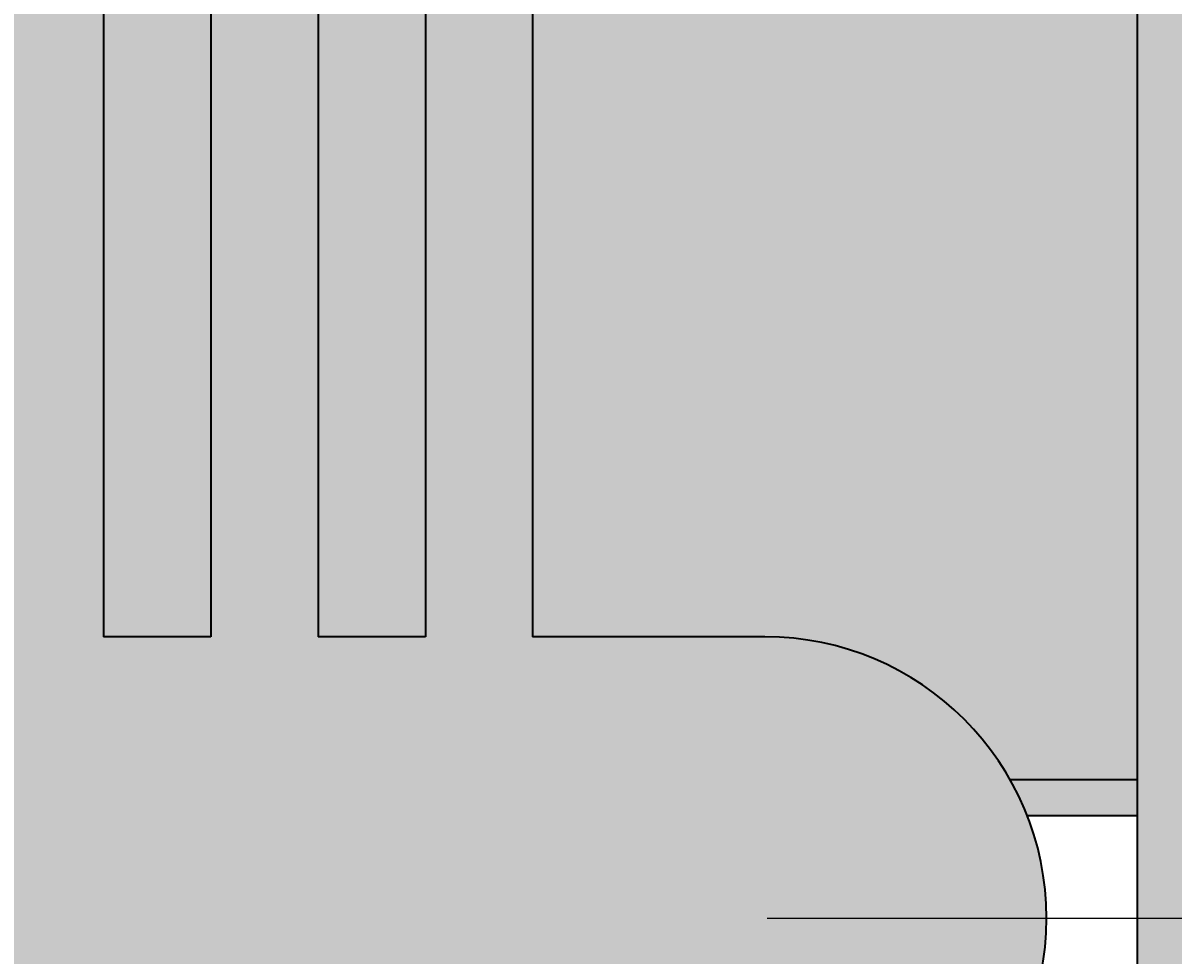
# Model space of a CAD drawing. Units: inches. Extents: x -1 to 292, y -3 to 199.
# Tile 26 of 52: x 148 to 181, y 42 to 68. Entities that reach past the tile are written whole.
import ezdxf

# ---------------------------------------------------------------- set-up
doc = ezdxf.new("R2010")
doc.units = ezdxf.units.IN
doc.header["$MEASUREMENT"] = 0
for name, color, linetype, lineweight in [('M-DIMS', 2, 'Continuous', 18), ('M-EQPM', 7, 'Continuous', 35), ('M-PATT', 8, 'Continuous', 13)]:
    doc.layers.add(name, color=color, linetype=linetype, lineweight=lineweight)
doc.styles.get("Standard").update_dxf_attribs({"font": 'arial.ttf'})
doc.dimstyles.get("Standard").update_dxf_attribs({"dimtxt": 0.18, "dimasz": 0.18, "dimexe": 0.18, "dimexo": 0.0625, "dimgap": 0.09, "dimtad": 0, "dimtih": 1, "dimtoh": 1, "dimdec": 4, "dimzin": 0, "dimdsep": 46, "dimtxsty": 'Standard', "dimcen": 0.09, "dimadec": 0, "dimazin": 0, "dimtfac": 1, "dimtdec": 4, "dimtofl": 0, "dimtmove": 0, "dimatfit": 3, "dimfxl": 1, "dimtolj": 1, "dimtzin": 0, "dimarcsym": 0})

# ---------------------------------------------------------------- blocks, each defined once
blk = doc.blocks.new('BOILER-TUBE')
for p, q in [((0, 40.63), (0, 0)), ((3, 40.63), (3, 0))]:
    blk.add_line(p, q)
for points in [[(0, 40.63), (3, 40.63)], [(3, 0), (0, 0)]]:
    blk.add_lwpolyline(points)
blk = doc.blocks.new('*D7')
at = {"layer": 'Defpoints', "color": 0, "transparency": 16777216}
for p in [(21.861, 54.582), (205.115, 54.582), (21.861, 39.982)]:
    blk.add_point(p, dxfattribs=at)
at = {"layer": 'M-DIMS', "color": 0, "lineweight": -2, "transparency": 16777216}
for p, q in [((21.861, 54.52), (21.861, 39.802)), ((205.115, 54.52), (205.115, 39.802)), ((22.041, 39.982), (113.033, 39.982)), ((204.935, 39.982), (113.944, 39.982))]:
    blk.add_line(p, q, dxfattribs=at)
at = {"layer": 'M-DIMS', "color": 0, "transparency": 16777216}
for points in [[(22.041, 40.012), (22.041, 39.952), (21.861, 39.982)], [(204.935, 40.012), (204.935, 39.952), (205.115, 39.982)]]:
    blk.add_solid(points, dxfattribs=at)
at = {"layer": 'M-DIMS', "color": 0, "transparency": 16777216, "insert": (113.488, 39.982), "char_height": 0.18, "attachment_point": 5}
blk.add_mtext('\\A1;183.25', dxfattribs=at)
blk = doc.blocks.new('*D10')
at = {"layer": 'Defpoints', "color": 0, "transparency": 16777216}
for p in [(169.176, 99.774), (169.176, 43.391), (292.04, 43.391)]:
    blk.add_point(p, dxfattribs=at)
at = {"layer": 'M-DIMS', "color": 0, "lineweight": -2, "transparency": 16777216}
for p, q in [((169.239, 99.774), (292.22, 99.774)), ((292.04, 99.594), (292.04, 71.764)), ((292.04, 43.571), (292.04, 71.4)), ((169.239, 43.391), (292.22, 43.391))]:
    blk.add_line(p, q, dxfattribs=at)
at = {"layer": 'M-DIMS', "color": 0, "transparency": 16777216}
for points in [[(292.01, 99.594), (292.07, 99.594), (292.04, 99.774)], [(292.01, 43.571), (292.07, 43.571), (292.04, 43.391)]]:
    blk.add_solid(points, dxfattribs=at)
at = {"layer": 'M-DIMS', "color": 0, "transparency": 16777216, "insert": (292.04, 71.582), "char_height": 0.18, "attachment_point": 5}
blk.add_mtext('\\A1;56.38', dxfattribs=at)

msp = doc.modelspace()

# ---------------------------------------------------------------- hatches: boundary and pattern name
at = {"layer": 'M-PATT'}
h = msp.add_hatch(color=256, dxfattribs=at)
h.set_gradient(color1=(0, 127, 0), color2=(0, 127, 0), tint=1, name='CYLINDER')
h.paths.add_polyline_path([(164.5186, 119.2985), (129.9293, 119.2985), (129.9293, 117.2985), (164.1897, 117.2985)])
h.paths.add_polyline_path([(181.5897, 119.2985), (164.5186, 119.2985), (164.1897, 117.2985), (179.5897, 117.2985), (179.5897, 107.8518), (181.5897, 109.1506)])
h.paths.add_polyline_path([(181.5897, 109.1506), (179.5897, 107.8518), (179.5897, 36.2698), (198.4159, 36.2698), (198.4159, 38.2698), (181.5897, 38.2698)])
h.paths.add_polyline_path([(115.4883, 126.765), (111.4883, 126.765), (111.4883, 114.6589), (115.4883, 114.6589)])
h.paths.add_polyline_path([(123.408, 119.2985), (115.4883, 119.2985), (115.4883, 117.2985), (123.408, 117.2985)])
h.paths.add_polyline_path([(115.4883, 112.6589), (111.4883, 112.6589), (111.4883, 106.9941), (115.4883, 106.9941)])
h.paths.add_polyline_path([(120.9032, 106.9941), (106.0735, 106.9941), (106.0735, 105.9941), (120.9032, 105.9941)])
h.paths.add_polyline_path([(236.4209, 117.5104), (234.9209, 117.5104), (234.9209, 97.1861), (236.4209, 97.1861)])
h.paths.add_polyline_path([(236.4209, 126.4904), (234.9209, 126.4904), (234.9209, 118.9331), (236.4209, 118.9331)])
h.paths.add_polyline_path([(244.9552, 125.7269), (242.9552, 125.7269), (242.9552, 116.8562), (244.9552, 116.8562)])
h.paths.add_polyline_path([(244.9552, 115.1721), (242.9552, 115.1721), (242.9552, 109.7385), (244.9552, 109.7385)])
h.paths.add_polyline_path([(248.4468, 109.7385), (239.4637, 109.7385), (239.4637, 109.4289), (248.4468, 109.4289)])
h = msp.add_hatch(color=256, dxfattribs=at)
h.set_gradient(color1=(237, 31, 36), color2=(242, 113, 114), tint=1, name='CYLINDER')
h.paths.add_polyline_path([(106.0735, 105.9941), (106.0735, 106.9941), (108.0603, 106.9941), (107.8488, 107.6501), (57.8007, 107.6501, 0.4142136), (49.9241, 99.7735), (52.3176, 101.3278), (55.0097, 99.7735), (57.4032, 101.3278), (60.0953, 99.7735), (62.4888, 101.3278), (65.1809, 99.7735), (67.5744, 101.3278), (70.2665, 99.7735), (72.66, 101.3278), (75.3521, 99.7735), (77.7456, 101.3278), (80.4377, 99.7735), (82.8312, 101.3278), (85.5233, 99.7735), (87.9168, 101.3278), (90.6089, 99.7735), (93.0024, 101.3278), (95.6945, 99.7735), (98.088, 101.3278), (100.7801, 99.7735), (103.1736, 101.3278), (105.8657, 99.7735), (108.2592, 101.3278), (110.9513, 99.7735), (113.3448, 101.3278), (116.0369, 99.7735), (118.4304, 101.3278), (121.1225, 99.7735), (123.516, 101.3278), (126.2082, 99.7735), (128.6016, 101.3278), (131.2938, 99.7735), (133.6872, 101.3278), (136.3794, 99.7735), (138.7728, 101.3278), (141.465, 99.7735), (143.8584, 101.3278), (146.5506, 99.7735), (148.944, 101.3278), (151.6362, 99.7735), (154.0296, 101.3278), (156.7218, 99.7735), (159.1152, 101.3278), (160.6222, 100.4578), (160.6222, 107.6501), (115.4883, 107.6501), (115.4883, 106.9941), (120.9032, 106.9941), (120.9032, 105.9941), (120.9032, 103.3981), (106.0735, 103.3981)])
h.paths.add_polyline_path([(169.176, 107.6501), (162.1623, 107.6501), (162.1623, 100.004), (164.2008, 101.3278), (166.893, 99.7735), (169.2864, 101.3278), (171.9786, 99.7735), (174.372, 101.3278), (177.0526, 99.7802, 0.4139642)])
h.paths.add_polyline_path([(111.4883, 107.6501), (107.8488, 107.6501), (108.0603, 106.9941), (111.4883, 106.9941)], flags=17)
h.paths.add_polyline_path([(61.6788, 91.897), (57.8007, 91.897, -0.1099266), (54.4604, 92.6403), (43.2011, 92.6403), (23.9502, 84.4688), (23.9502, 58.376), (43.2011, 47.2615), (50.9409, 47.2615, -0.2705926), (57.8007, 51.2672), (61.6788, 51.2672)])
h.paths.add_polyline_path([(73.6788, 91.897), (70.6788, 91.897), (70.6788, 51.2672), (73.6788, 51.2672)])
h.paths.add_polyline_path([(79.6788, 91.897), (76.6788, 91.897), (76.6788, 51.2672), (79.6788, 51.2672)])
h.paths.add_polyline_path([(67.6788, 91.897), (64.6788, 91.897), (64.6788, 51.2672), (67.6788, 51.2672)])
h.paths.add_polyline_path([(101.6788, 91.897), (82.6788, 91.897), (82.6788, 51.2672), (101.6788, 51.2672)])
h.paths.add_polyline_path([(107.6788, 91.897), (104.6788, 91.897), (104.6788, 51.2672), (107.6788, 51.2672)])
h.paths.add_polyline_path([(113.6788, 91.897), (110.6788, 91.897), (110.6788, 51.2672), (113.6788, 51.2672)])
h.paths.add_polyline_path([(119.6788, 91.897), (116.6788, 91.897), (116.6788, 51.2672), (119.6788, 51.2672)])
h.paths.add_polyline_path([(141.6788, 91.897), (122.6788, 91.897), (122.6788, 51.2672), (141.6788, 51.2672)])
h.paths.add_polyline_path([(147.6788, 91.897), (144.6788, 91.897), (144.6788, 51.2672), (147.6788, 51.2672)])
h.paths.add_polyline_path([(153.6788, 91.897), (150.6788, 91.897), (150.6788, 51.2672), (153.6788, 51.2672)])
h.paths.add_polyline_path([(159.6788, 91.897), (156.6788, 91.897), (156.6788, 51.2672), (159.6788, 51.2672)])
h.paths.add_polyline_path([(179.5897, 92.6403), (172.5163, 92.6403, -0.1099266), (169.176, 91.897), (162.6788, 91.897), (162.6788, 51.2672), (169.176, 51.2672, -0.2705926), (176.0358, 47.2615), (179.5897, 47.2615)])
h.paths.add_polyline_path([(203.0265, 84.4688), (183.7755, 92.6403), (181.5897, 92.6403), (181.5897, 47.2615), (183.7755, 47.2615), (203.0265, 58.376)])
h.paths.add_polyline_path([(184.4188, 61.52), (200.7224, 61.52), (200.7224, 77.7532), (184.4188, 77.7532)], flags=24)
h = msp.add_hatch(color=256, dxfattribs=at)
h.set_gradient(color1=(0, 255, 255), color2=(0, 255, 255), tint=1)
h.paths.add_polyline_path([(75.3521, 99.7735), (72.66, 101.3278), (70.2665, 99.7735), (67.5744, 101.3278), (65.1809, 99.7735), (62.4888, 101.3278), (60.0953, 99.7735), (57.4032, 101.3278), (55.0097, 99.7735), (52.3176, 101.3278), (49.9241, 99.7735, 0.4142136), (57.8007, 91.897), (61.6788, 91.897), (61.6788, 51.2672), (57.8007, 51.2672, 0.8088808), (54.5813, 36.2021), (65.0947, 51.2672), (64.6788, 51.2672), (64.6788, 91.897), (67.6788, 91.897), (67.6788, 51.2672), (65.0947, 51.2672), (54.5813, 36.2021, 0.1056561), (57.8007, 35.5141), (169.176, 35.5141, 1), (169.176, 51.2672), (162.6788, 51.2672), (162.6788, 91.897), (169.176, 91.897, 0.4144629), (177.0526, 99.7802), (174.372, 101.3278), (171.9786, 99.7735), (169.2864, 101.3278), (166.893, 99.7735), (164.2008, 101.3278), (162.1623, 100.004), (162.1623, 96.1027), (160.6222, 96.1027), (160.6222, 100.4578), (159.1152, 101.3278), (156.7218, 99.7735), (154.0296, 101.3278), (151.6362, 99.7735), (148.944, 101.3278), (146.5506, 99.7735), (143.8584, 101.3278), (141.465, 99.7735), (138.7728, 101.3278), (136.3794, 99.7735), (133.6872, 101.3278), (131.2938, 99.7735), (128.6016, 101.3278), (126.2082, 99.7735), (123.516, 101.3278), (121.1225, 99.7735), (118.4304, 101.3278), (116.0369, 99.7735), (113.3448, 101.3278), (110.9513, 99.7735), (108.2592, 101.3278), (105.8657, 99.7735), (103.1736, 101.3278), (100.7801, 99.7735), (98.088, 101.3278), (95.6945, 99.7735), (93.0024, 101.3278), (90.6089, 99.7735), (87.9168, 101.3278), (85.5233, 99.7735), (82.8312, 101.3278), (80.4377, 99.7735), (77.7456, 101.3278)])
h.paths.add_polyline_path([(79.6788, 91.897), (79.6788, 51.2672), (76.6788, 51.2672), (76.6788, 91.897)], flags=16)
h.paths.add_polyline_path([(73.6788, 91.897), (73.6788, 51.2672), (70.6788, 51.2672), (70.6788, 91.897)], flags=16)
h.paths.add_polyline_path([(82.6788, 91.897), (101.6788, 91.897), (101.6788, 51.2672), (82.6788, 51.2672)], flags=16)
h.paths.add_polyline_path([(104.6788, 91.897), (107.6788, 91.897), (107.6788, 51.2672), (104.6788, 51.2672)], flags=16)
h.paths.add_polyline_path([(110.6788, 91.897), (113.6788, 91.897), (113.6788, 51.2672), (110.6788, 51.2672)], flags=16)
h.paths.add_polyline_path([(116.6788, 91.897), (119.6788, 91.897), (119.6788, 51.2672), (116.6788, 51.2672)], flags=16)
h.paths.add_polyline_path([(122.6788, 91.897), (141.6788, 91.897), (141.6788, 51.2672), (144.6788, 51.2672), (144.6788, 91.897), (147.6788, 91.897), (147.6788, 51.2672), (122.6788, 51.2672)], flags=16)
h.paths.add_polyline_path([(150.6788, 91.897), (153.6788, 91.897), (153.6788, 51.2672), (150.6788, 51.2672)], flags=16)
h.paths.add_polyline_path([(156.6788, 91.897), (159.6788, 91.897), (159.6788, 51.2672), (156.6788, 51.2672)], flags=16)
h = msp.add_hatch(color=256, dxfattribs=at)
h.set_gradient(color1=(76, 38, 47), color2=(76, 38, 47), tint=1, name='CYLINDER')
h.paths.add_polyline_path([(40.8628, 91.6478), (40.3591, 92.5203), (23.9502, 85.5552), (23.9502, 84.4688)])
h.paths.add_polyline_path([(52.8586, 93.6403), (42.9977, 93.6403), (40.3591, 92.5203), (40.8628, 91.6478), (43.2011, 92.6403), (54.4604, 92.6403, -0.0601508)])
h.paths.add_polyline_path([(23.9502, 88.5821), (21.8612, 88.5821), (21.8612, 54.5821), (23.9502, 54.5821)])
h.paths.add_polyline_path([(23.9502, 58.376), (23.9502, 57.2213), (42.9332, 46.2615), (50.4659, 46.2615, -0.0351813), (50.9409, 47.2615), (43.2011, 47.2615)])
h.paths.add_polyline_path([(179.5897, 93.6403), (174.1181, 93.6403, -0.0601508), (172.5163, 92.6403), (179.5897, 92.6403)])
h.paths.add_polyline_path([(183.979, 93.6403), (181.5897, 93.6403), (181.5897, 92.6403), (183.7755, 92.6403), (203.0265, 84.4688), (203.0265, 85.5552)])
h.paths.add_polyline_path([(205.1155, 88.5821), (203.0265, 88.5821), (203.0265, 54.5821), (205.1155, 54.5821)])
h.paths.add_polyline_path([(203.0265, 57.2213), (203.0265, 58.376), (183.7755, 47.2615), (181.5897, 47.2615), (181.5897, 46.2615), (184.0435, 46.2615)])
h.paths.add_polyline_path([(179.5897, 47.2615), (176.0358, 47.2615, -0.0351813), (176.5107, 46.2615), (179.5897, 46.2615)])

# ---------------------------------------------------------------- linework, layer by layer
at = {"layer": 'M-EQPM'}
msp.add_line((162.6788, 91.897), (162.6788, 51.2672), dxfattribs=at)
for points in [[(129.9293, 117.2985), (179.5897, 117.2985), (179.5897, 36.2698)], [(179.5897, 47.2615), (176.0358, 47.2615)], [(179.5897, 46.2615), (176.5107, 46.2615)]]:
    msp.add_lwpolyline(points, dxfattribs=at)
msp.add_lwpolyline([(61.6788, 51.2672), (57.8007, 51.2672, 1), (57.8007, 35.5141), (169.176, 35.5141, 1), (169.176, 51.2672), (162.6788, 51.2672)], format="xyb", dxfattribs=at)

# ---------------------------------------------------------------- block references
for p in [(150.679, 51.267), (156.679, 51.267)]:
    msp.add_blockref('BOILER-TUBE', p, dxfattribs=at)

# ---------------------------------------------------------------- dimensions: what is measured, and where the dimension line sits
at = {"layer": 'M-DIMS'}
for base, p1, p2, angle, picture, middle in [((292.0399, 43.3906), (169.176, 99.7735), (169.176, 43.3906), 90, '*D10', (292.0399, 71.5821)), ((21.8612, 39.9821), (205.1155, 54.5821), (21.8612, 54.5821), 180, '*D7', (113.4883, 39.9821))]:
    dim = msp.add_linear_dim(base=base, p1=p1, p2=p2, angle=angle, dimstyle='Standard', override={"dimdec": 2, "dimlfac": 1, "dimrnd": 0, "dimzin": 0, "dimdsep": 46, "dimlunit": 2}, dxfattribs=at)
    dim.commit()
    dim.dimension.update_dxf_attribs({"geometry": picture, "text_midpoint": middle})

doc.saveas('drawing.dxf')
